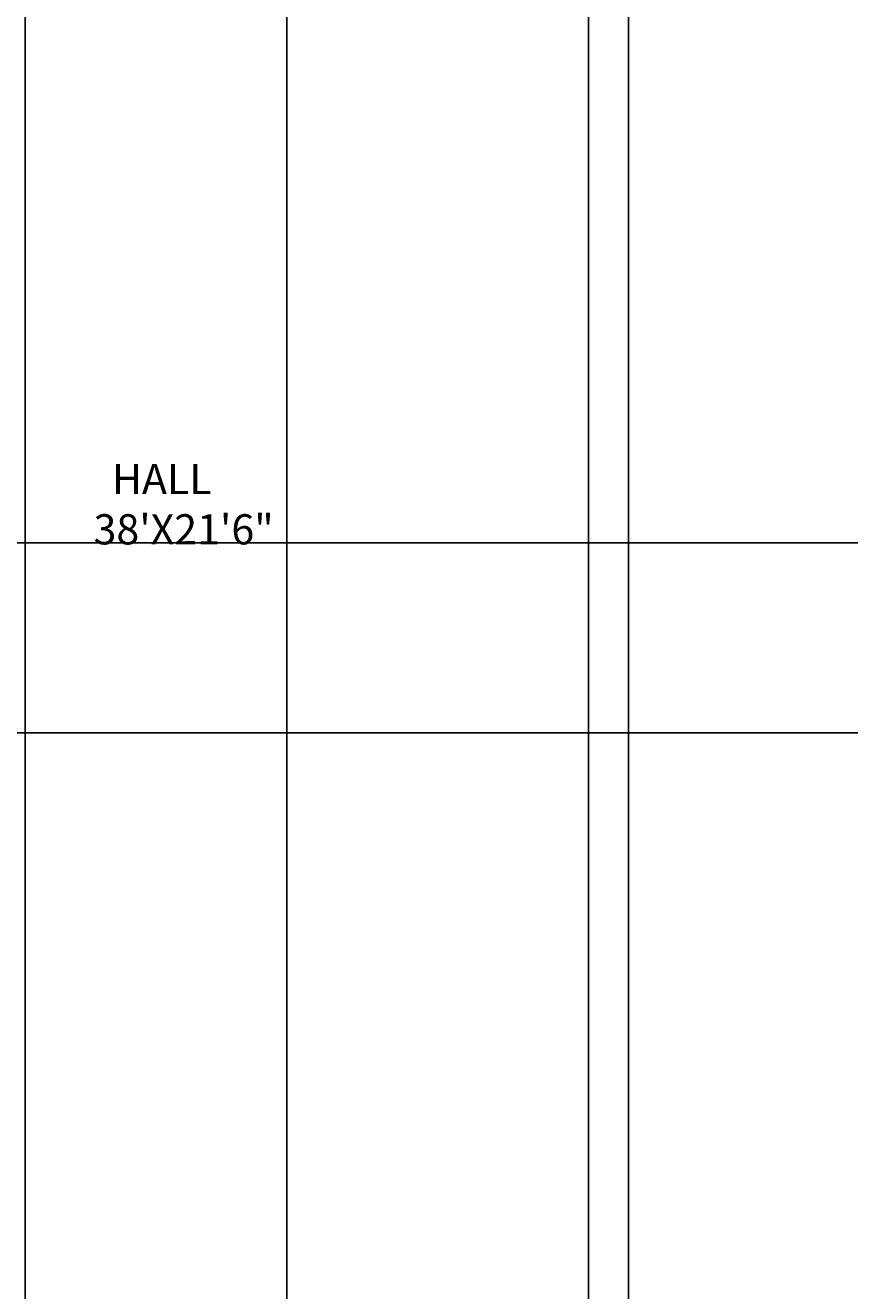
# Model space of a CAD drawing. Units: inches. Extents: x 318 to 927, y -1130 to 13.
# Tile 9 of 17: x 599 to 763, y -692 to -440. Entities that reach past the tile are written whole.
import ezdxf

# ---------------------------------------------------------------- set-up
doc = ezdxf.new("R2010")
doc.units = ezdxf.units.IN
doc.header["$MEASUREMENT"] = 0
doc.layers.add('A-ANNO-DIMS', color=1, linetype='Continuous', lineweight=18)
doc.layers.add('A-AREA-IDEN', color=8, linetype='Continuous', lineweight=18)
doc.styles.get("Standard").update_dxf_attribs({"font": 'arial.ttf'})
doc.dimstyles.get("Standard").update_dxf_attribs({"dimtxt": 0.18, "dimasz": 0.18, "dimexe": 0.18, "dimexo": 0.0625, "dimgap": 0.09, "dimtad": 0, "dimtih": 1, "dimtoh": 1, "dimdec": 1, "dimzin": 0, "dimdsep": 46, "dimlunit": 4, "dimtxsty": 'Standard', "dimcen": 0.09, "dimadec": 0, "dimazin": 0, "dimtfac": 1, "dimtdec": 1, "dimtofl": 0, "dimtmove": 0, "dimatfit": 3, "dimfxl": 1, "dimtolj": 1, "dimtzin": 0, "dimarcsym": 0})

# ---------------------------------------------------------------- blocks, each defined once
blk = doc.blocks.new('*D27')
at = {"layer": 'A-ANNO-DIMS', "color": 0, "lineweight": -2, "transparency": 16777216}
for p, q in [((598.89, -309.98), (598.89, -1124.59)), ((718.89, -309.98), (718.89, -1124.59)), ((599.07, -1124.41), (658.5, -1124.41)), ((718.71, -1124.41), (659.28, -1124.41))]:
    blk.add_line(p, q, dxfattribs=at)
at = {"layer": 'A-ANNO-DIMS', "color": 0, "transparency": 16777216}
for points in [[(599.07, -1124.38), (599.07, -1124.44), (598.89, -1124.41)], [(718.71, -1124.38), (718.71, -1124.44), (718.89, -1124.41)]]:
    blk.add_solid(points, dxfattribs=at)
at = {"layer": 'Defpoints', "color": 0, "transparency": 16777216}
for p in [(598.89, -309.91), (718.89, -309.91), (718.89, -1124.41)]:
    blk.add_point(p, dxfattribs=at)
at = {"layer": 'A-ANNO-DIMS', "color": 0, "transparency": 16777216, "insert": (658.89, -1124.41), "char_height": 0.18, "attachment_point": 5}
blk.add_mtext('\\A1;10\'-0"', dxfattribs=at)
blk = doc.blocks.new('*D28')
at = {"layer": 'A-ANNO-DIMS', "color": 0, "lineweight": -2, "transparency": 16777216}
for p, q in [((650.89, -1033.85), (650.89, -25.23)), ((651.07, -25.41), (680.57, -25.41)), ((710.71, -25.41), (681.22, -25.41)), ((710.89, -1033.85), (710.89, -25.23))]:
    blk.add_line(p, q, dxfattribs=at)
at = {"layer": 'A-ANNO-DIMS', "color": 0, "transparency": 16777216}
for points in [[(651.07, -25.38), (651.07, -25.44), (650.89, -25.41)], [(710.71, -25.38), (710.71, -25.44), (710.89, -25.41)]]:
    blk.add_solid(points, dxfattribs=at)
at = {"layer": 'Defpoints', "color": 0, "transparency": 16777216}
for p in [(710.89, -25.41), (650.89, -1033.91), (710.89, -1033.91)]:
    blk.add_point(p, dxfattribs=at)
at = {"layer": 'A-ANNO-DIMS', "color": 0, "transparency": 16777216, "insert": (680.89, -25.41), "char_height": 0.18, "attachment_point": 5}
blk.add_mtext('\\A1;5\'-0"', dxfattribs=at)
blk = doc.blocks.new('*D29')
at = {"layer": 'A-ANNO-DIMS', "color": 0, "lineweight": -2, "transparency": 16777216}
for p, q in [((598.89, -1033.85), (598.89, -25.23)), ((599.07, -25.41), (624.56, -25.41)), ((650.71, -25.41), (625.23, -25.41)), ((650.89, -1033.85), (650.89, -25.23))]:
    blk.add_line(p, q, dxfattribs=at)
at = {"layer": 'A-ANNO-DIMS', "color": 0, "transparency": 16777216}
for points in [[(599.07, -25.38), (599.07, -25.44), (598.89, -25.41)], [(650.71, -25.38), (650.71, -25.44), (650.89, -25.41)]]:
    blk.add_solid(points, dxfattribs=at)
at = {"layer": 'Defpoints', "color": 0, "transparency": 16777216}
for p in [(650.89, -25.41), (598.89, -1033.91), (650.89, -1033.91)]:
    blk.add_point(p, dxfattribs=at)
at = {"layer": 'A-ANNO-DIMS', "color": 0, "transparency": 16777216, "insert": (624.89, -25.41), "char_height": 0.18, "attachment_point": 5}
blk.add_mtext('\\A1;4\'-4"', dxfattribs=at)
blk = doc.blocks.new('*D41')
at = {"layer": 'A-ANNO-DIMS', "color": 0, "lineweight": -2, "transparency": 16777216}
for p, q in [((790.59, -543.15), (331.21, -543.15)), ((331.39, -543.33), (331.39, -561.86)), ((331.39, -580.75), (331.39, -562.22)), ((790.59, -580.93), (331.21, -580.93))]:
    blk.add_line(p, q, dxfattribs=at)
at = {"layer": 'A-ANNO-DIMS', "color": 0, "transparency": 16777216}
for points in [[(331.36, -543.33), (331.42, -543.33), (331.39, -543.15)], [(331.36, -580.75), (331.42, -580.75), (331.39, -580.93)]]:
    blk.add_solid(points, dxfattribs=at)
at = {"layer": 'Defpoints', "color": 0, "transparency": 16777216}
for p in [(790.65, -543.15), (331.39, -580.93), (790.65, -580.93)]:
    blk.add_point(p, dxfattribs=at)
at = {"layer": 'A-ANNO-DIMS', "color": 0, "transparency": 16777216, "insert": (331.39, -562.04), "char_height": 0.18, "attachment_point": 5}
blk.add_mtext('\\A1;3\'-2"', dxfattribs=at)

msp = doc.modelspace()

# ---------------------------------------------------------------- texts
at = {"layer": 'A-AREA-IDEN', "insert": (601.47, -527.43), "char_height": 6, "attachment_point": 1}
msp.add_mtext_dynamic_manual_height_columns('        HALL\\P      38\'X21\'6"', width=56.2093, gutter_width=1, heights=[0], dxfattribs=at)

# ---------------------------------------------------------------- dimensions: what is measured, and where the dimension line sits
at = {"layer": 'A-ANNO-DIMS'}
for base, p1, p2, picture, middle in [((650.89, -25.41), (598.89, -1033.91), (650.89, -1033.91), '*D29', (624.89, -25.41)), ((710.89, -25.41), (650.89, -1033.91), (710.89, -1033.91), '*D28', (680.89, -25.41)), ((718.89, -1124.41), (598.89, -309.91), (718.89, -309.91), '*D27', (658.89, -1124.41))]:
    dim = msp.add_linear_dim(base=base, p1=p1, p2=p2, dimstyle='Standard', override={"dimdec": 1, "dimlfac": 1, "dimrnd": 0, "dimzin": 1, "dimdsep": 46, "dimlunit": 4, "dimfrac": 2}, dxfattribs=at)
    dim.commit()
    dim.dimension.update_dxf_attribs({"geometry": picture, "text_midpoint": middle})
dim = msp.add_linear_dim(base=(331.39, -580.93), p1=(790.65, -543.15), p2=(790.65, -580.93), angle=90, dimstyle='Standard', override={"dimdec": 1, "dimlfac": 1, "dimrnd": 0, "dimzin": 1, "dimdsep": 46, "dimlunit": 4, "dimfrac": 2}, dxfattribs=at)
dim.commit()
dim.dimension.update_dxf_attribs({"geometry": '*D41', "text_midpoint": (331.39, -562.04)})

doc.saveas('drawing.dxf')
